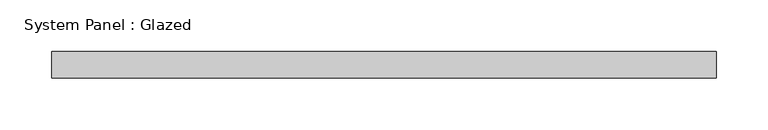
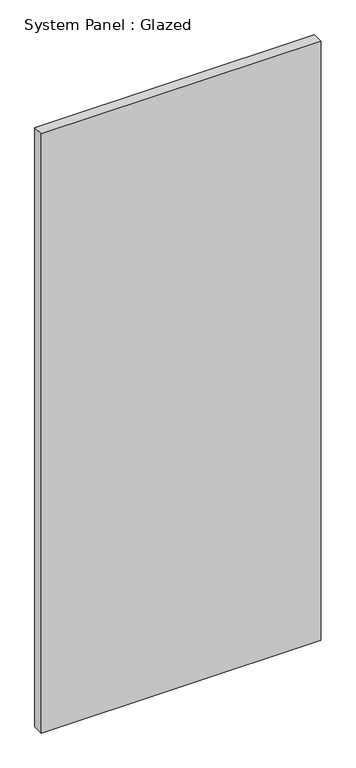
"""IFC4 building model written with IfcOpenShell, lengths in millimetres: plate geometry, System Panel : Glazed."""

from ifc_helpers import new_model, si_unit, origin, origin_with_axes, place, context, project, spatial, polyline, outline, extrude, source, transform, mapped, element, save


def system_panel_glazed_ddf70934(model_context):
    return source(origin(), model_context, "Body", "SweptSolid", [
        extrude(outline(polyline([(320.675, 19.05), (-320.675, 19.05), (-320.675, 44.45), (320.675, 44.45), (320.675, 19.05)])), origin_with_axes(), (0.0, 0.0, 1.0), 1451.2793787),
    ])


if __name__ == "__main__":
    model = new_model("IFC4")
    model_context = context("Model", 3, world=origin())
    ifc_project = project(units=[si_unit("LENGTHUNIT", "METRE", prefix="MILLI")], contexts=[model_context])
    site = spatial("IfcSite", under=ifc_project)
    building = spatial("IfcBuilding", under=site)
    placement = place(None, origin())
    system_panel_glazed_shape = system_panel_glazed_ddf70934(model_context)
    element("IfcPlate", 1, ObjectType="System Panel : Glazed", at=placement, inside=building, context=model_context, shape_type="MappedRepresentation", body=[
        mapped(system_panel_glazed_shape, transform((0.0, 0.0, 0.0), x_axis=(1.0, 0.0, 0.0), y_axis=(0.0, 1.0, 0.0), z_axis=(0.0, 0.0, 1.0))),
    ])
    save(model, "model.ifc")

# Revit data of these elements
# Type "System Panel : Glazed"
#   Construction Type Id = "GSP4R"
#   Analytic Construction = "1/8 in Pilkington single glazing"
#   Visual Light Transmittance = 0.9
#   Solar Heat Gain Coefficient = 0.86
#   Heat Transfer Coefficient (U) = 1.18115 BTU/(h·ft²·°F)
#   Define Thermal Properties by = 1
# Element 1 (IfcPlate, "System Panel : Glazed")
#   Materials on its faces: "Glass"
# Materials
#   "Glass": class "Glass", colour RGB 0 128 192, transparency 0.75, Description = "Soda Lime Glass", Cost = 0
